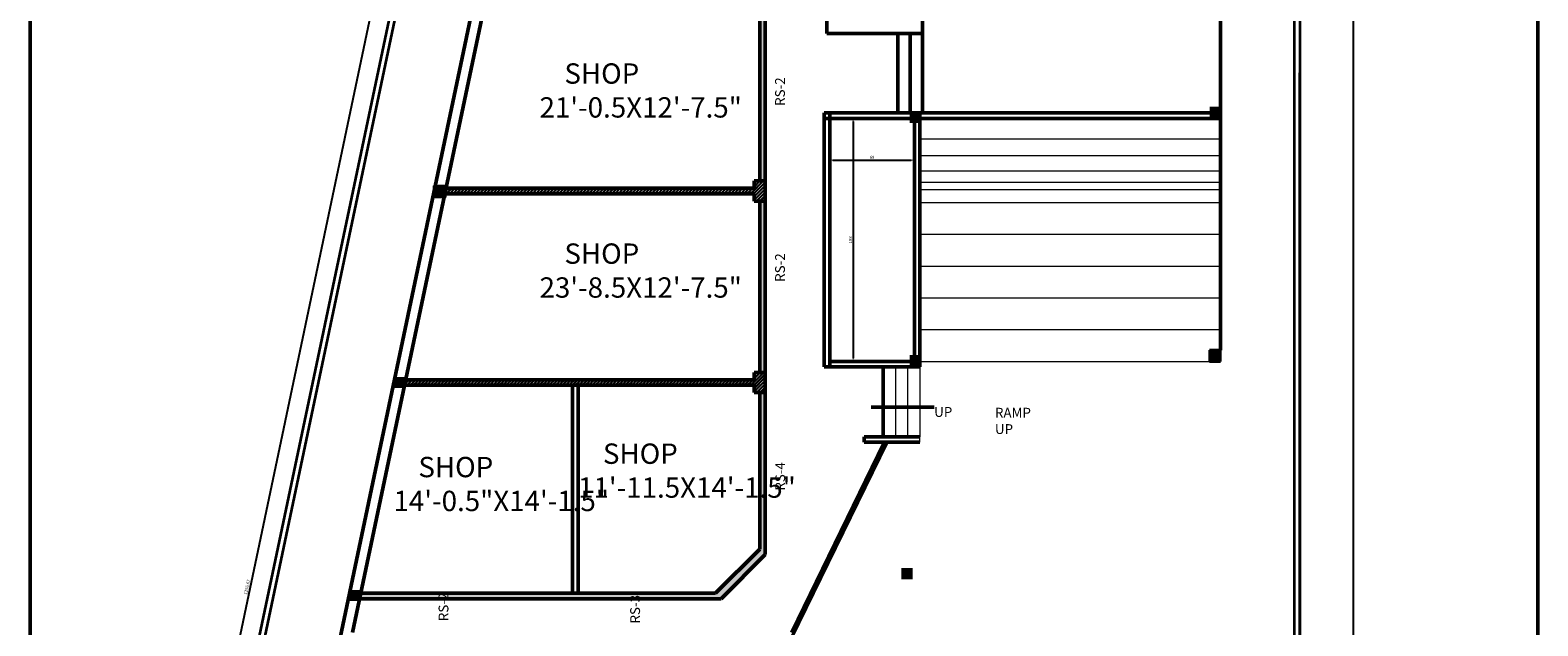
# Model space of a CAD drawing. Units: millimetres. Extents: x 2134 to 3363, y 1052 to 3233.
# Tile 5 of 11: x 2134 to 3363, y 1782 to 2268. Entities that reach past the tile are written whole.
import ezdxf

# ---------------------------------------------------------------- set-up
doc = ezdxf.new("R2010")
doc.units = ezdxf.units.MM
for name, color, linetype, lineweight in [('A-ANNO-DIMS', 2, 'Continuous', 18), ('A-ANNO-TEXT', 7, 'Continuous', 18), ('A-ANNO-TTLB', 7, 'Continuous', 50), ('A-AREA-IDEN', 3, 'Continuous', 18), ('A-COLS', 1, 'Continuous', 35), ('A-FLOR-STRS', 3, 'Continuous', 18), ('A-WALL', 7, 'Continuous', 50), ('A-WALL-PATT', 8, 'Continuous', 13), ('C-PROP', 6, 'Continuous', 35)]:
    doc.layers.add(name, color=color, linetype=linetype, lineweight=lineweight)
doc.styles.get("Standard").update_dxf_attribs({"font": 'arial.ttf'})
doc.styles.add('YQ_DIM', font='SUPEROS.SHX', dxfattribs={"width": 0.8, "bigfont": 'HZDX.SHX'})
doc.dimstyles.new('ISO-25', dxfattribs={"dimtxt": 2.5, "dimasz": 2.5, "dimexe": 1.25, "dimexo": 0.625, "dimtad": 1, "dimtxsty": 'Standard', "dimcen": 2.5, "dimadec": 0, "dimazin": 0, "dimtfac": 1, "dimtmove": 0, "dimatfit": 3, "dimfxl": 1, "dimarcsym": 0})

# ---------------------------------------------------------------- blocks, each defined once
blk = doc.blocks.new('*D8')
at = {"layer": 'A-ANNO-DIMS', "color": 0, "lineweight": -2, "transparency": 16777216}
for p, q in [((2442.4, 2425.8), (2184.5, 1201)), ((2457.7, 2425.1), (2441.7, 2428.5)), ((2198.8, 1195.4), (2182.8, 1198.8))]:
    blk.add_line(p, q, dxfattribs=at)
at = {"layer": 'A-ANNO-DIMS', "color": 0, "transparency": 16777216}
for points in [[(2442, 2425.9), (2442.8, 2425.7), (2442.9, 2428.3)], [(2184.1, 1201.1), (2185, 1200.9), (2184, 1198.5)]]:
    blk.add_solid(points, dxfattribs=at)
at = {"layer": 'Defpoints', "color": 0, "transparency": 16777216}
for p in [(2458.4, 2425), (2184, 1198.5), (2199.5, 1195.3)]:
    blk.add_point(p, dxfattribs=at)
at = {"layer": 'A-ANNO-DIMS', "color": 0, "transparency": 16777216, "insert": (2311.4, 1813.8), "char_height": 2.5, "attachment_point": 5, "rotation": 78.1108}
blk.add_mtext('1256,67', dxfattribs=at)
blk = doc.blocks.new('*D9')
at = {"layer": 'A-ANNO-DIMS', "color": 0, "lineweight": -2, "transparency": 16777216}
for p, q in [((3169.5, 3063.8), (3213.5, 3063.8)), ((3212.2, 3061.3), (3212.2, 1770.3)), ((3169.5, 1767.8), (3213.5, 1767.8))]:
    blk.add_line(p, q, dxfattribs=at)
at = {"layer": 'A-ANNO-DIMS', "color": 0, "transparency": 16777216}
for points in [[(3211.8, 3061.3), (3212.6, 3061.3), (3212.2, 3063.8)], [(3211.8, 1770.3), (3212.6, 1770.3), (3212.2, 1767.8)]]:
    blk.add_solid(points, dxfattribs=at)
at = {"layer": 'Defpoints', "color": 0, "transparency": 16777216}
for p in [(3168.8, 3063.8), (3168.8, 1767.8), (3212.2, 1767.8)]:
    blk.add_point(p, dxfattribs=at)
at = {"layer": 'A-ANNO-DIMS', "color": 0, "transparency": 16777216, "insert": (3210.3, 2415.8), "char_height": 2.5, "attachment_point": 5, "rotation": 90}
blk.add_mtext('1296', dxfattribs=at)
blk = doc.blocks.new('*D13')
at = {"layer": 'A-ANNO-DIMS', "color": 0, "lineweight": -2, "transparency": 16777216}
for p, q in [((2785.8, 2162.4), (2785.8, 2163)), ((2854.8, 2162.4), (2854.8, 2163)), ((2788.3, 2161.8), (2852.3, 2161.8))]:
    blk.add_line(p, q, dxfattribs=at)
at = {"layer": 'A-ANNO-DIMS', "color": 0, "transparency": 16777216}
for points in [[(2788.3, 2162.2), (2788.3, 2161.3), (2785.8, 2161.8)], [(2852.3, 2162.2), (2852.3, 2161.3), (2854.8, 2161.8)]]:
    blk.add_solid(points, dxfattribs=at)
at = {"layer": 'Defpoints', "color": 0, "transparency": 16777216}
for p in [(2785.8, 2161.8), (2854.8, 2161.8), (2854.8, 2161.8)]:
    blk.add_point(p, dxfattribs=at)
at = {"layer": 'A-ANNO-DIMS', "color": 0, "transparency": 16777216, "insert": (2820.3, 2163.7), "char_height": 2.5, "attachment_point": 5}
blk.add_mtext('69', dxfattribs=at)
blk = doc.blocks.new('*D14')
at = {"layer": 'A-ANNO-DIMS', "color": 0, "lineweight": -2, "transparency": 16777216}
for p, q in [((2804.4, 2195.8), (2806.2, 2195.8)), ((2804.9, 2193.3), (2804.9, 2000.3)), ((2809.9, 1997.8), (2803.7, 1997.8))]:
    blk.add_line(p, q, dxfattribs=at)
at = {"layer": 'A-ANNO-DIMS', "color": 0, "transparency": 16777216}
for points in [[(2804.5, 2193.3), (2805.3, 2193.3), (2804.9, 2195.8)], [(2804.5, 2000.3), (2805.3, 2000.3), (2804.9, 1997.8)]]:
    blk.add_solid(points, dxfattribs=at)
at = {"layer": 'Defpoints', "color": 0, "transparency": 16777216}
for p in [(2803.8, 2195.8), (2804.9, 1997.8), (2810.6, 1997.8)]:
    blk.add_point(p, dxfattribs=at)
at = {"layer": 'A-ANNO-DIMS', "color": 0, "transparency": 16777216, "insert": (2803, 2096.8), "char_height": 2.5, "attachment_point": 5, "rotation": 90}
blk.add_mtext('198', dxfattribs=at)
blk = doc.blocks.new('*D6')
at = {"layer": 'A-ANNO-DIMS', "color": 0, "lineweight": -2, "transparency": 16777216}
blk.add_arc((2458.4, 2425), 20.3, 94.064, 251.0467, dxfattribs=at)
at = {"layer": 'A-ANNO-DIMS', "color": 0, "transparency": 16777216}
for points in [[(2456.9, 2445.7), (2456.9, 2444.8), (2459.4, 2445.3)], [(2451.9, 2406.2), (2451.7, 2405.4), (2454.2, 2405.2)]]:
    blk.add_solid(points, dxfattribs=at)
at = {"layer": 'Defpoints', "color": 0, "transparency": 16777216}
for p in [(2491.8, 3063.8), (2441.9, 2436.9), (2458.4, 2425), (2458.4, 2425), (2197.1, 1183.9)]:
    blk.add_point(p, dxfattribs=at)
at = {"layer": 'A-ANNO-DIMS', "color": 0, "transparency": 16777216, "insert": (2436.4, 2427.9), "char_height": 2.5, "attachment_point": 5, "rotation": 82.5554}
blk.add_mtext('171°', dxfattribs=at)

msp = doc.modelspace()

# ---------------------------------------------------------------- hatches: boundary and pattern name
at = {"layer": 'A-COLS'}
h = msp.add_hatch(color=256, dxfattribs=at)
h.dxf.hatch_style = 1
h.paths.add_polyline_path([(2859.858, 2200.875), (2850.858, 2200.875), (2850.858, 2191.875), (2859.858, 2191.875)])
h = msp.add_hatch(color=256, dxfattribs=at)
h.dxf.hatch_style = 1
h.paths.add_polyline_path([(3104.339, 2205.375), (3095.339, 2205.375), (3095.339, 2196.375), (3104.339, 2196.375)])
h = msp.add_hatch(color=256, dxfattribs=at)
h.dxf.hatch_style = 1
h.paths.add_polyline_path([(2472.483, 2140.686), (2464.415, 2140.686), (2463.483, 2136.26), (2463.483, 2131.686), (2471.635, 2131.686), (2472.483, 2135.714)])
h = msp.add_hatch(color=256, dxfattribs=at)
h.dxf.hatch_style = 1
h.paths.add_polyline_path([(2859.858, 2002.875), (2850.858, 2002.875), (2850.858, 1993.875), (2859.858, 1993.875)])
h = msp.add_hatch(color=256, dxfattribs=at)
h.dxf.hatch_style = 1
h.paths.add_polyline_path([(3104.339, 2006.774), (3095.339, 2006.774), (3095.339, 1997.774), (3104.339, 1997.774)])
h = msp.add_hatch(color=256, dxfattribs=at)
h.dxf.hatch_style = 1
h.paths.add_polyline_path([(2440.045, 1985.133), (2431.045, 1985.133), (2431.045, 1976.133), (2440.045, 1976.133)])
h = msp.add_hatch(color=256, dxfattribs=at)
h.dxf.hatch_style = 1
h.paths.add_polyline_path([(2853.256, 1829.254), (2844.256, 1829.254), (2844.256, 1820.254), (2853.256, 1820.254)])
h = msp.add_hatch(color=256, dxfattribs=at)
h.dxf.hatch_style = 1
h.paths.add_polyline_path([(2403.25, 1811.556), (2394.25, 1811.556), (2394.25, 1802.556), (2403.25, 1802.556)])
at = {"layer": 'A-WALL-PATT'}
h = msp.add_hatch(color=256, dxfattribs=at)
h.dxf.hatch_style = 1
h.paths.add_polyline_path([(2733.282, 2279.774), (2728.782, 2279.774), (2728.782, 2144.774), (2733.282, 2144.774)])
h.paths.add_polyline_path([(2733.282, 2435.778), (2728.782, 2435.778), (2728.782, 2296.274), (2733.282, 2296.274)])
h.paths.add_polyline_path([(2733.282, 2128.274), (2728.782, 2128.274), (2728.782, 1988.794), (2733.282, 1988.794)])
h.paths.add_polyline_path([(2733.282, 1972.299), (2728.782, 1972.299), (2728.782, 1844.774), (2692.782, 1808.774), (2403.682, 1808.774), (2402.735, 1804.274), (2697.282, 1804.274), (2733.282, 1840.274)])
h.paths.add_polyline_path([(2733.282, 2591.847), (2728.782, 2591.847), (2728.782, 2452.274), (2733.282, 2452.276)])
h.paths.add_polyline_path([(2733.282, 2747.554), (2728.782, 2747.554), (2728.782, 2608.342), (2733.282, 2608.342)])
h.paths.add_polyline_path([(2733.282, 2843.718), (2728.782, 2843.718), (2728.782, 2764.049), (2733.282, 2764.049)])
h.paths.add_polyline_path([(2733.282, 3012.274), (2728.782, 3012.274), (2728.782, 2860.213), (2733.282, 2860.213)])
h = msp.add_hatch(dxfattribs=at)
h.set_pattern_fill('ANSI32', color=256, scale=0.2)
h.set_pattern_definition([(45, (2052.4981, 1503.6934), (-1.3470384, 1.3470384), []), (45, (2053.3961, 1503.6934), (-1.3470384, 1.3470384), [])])
h.paths.add_polyline_path([(2733.282, 2144.774), (2728.782, 2144.774), (2728.782, 2144.769), (2724.282, 2144.769), (2724.282, 2138.774), (2473.126, 2138.774), (2472.179, 2134.274), (2724.282, 2134.274), (2724.282, 2128.274), (2728.782, 2128.274), (2733.282, 2128.274)])
h.paths.add_polyline_path([(2733.282, 2608.342), (2724.282, 2608.342), (2724.282, 2602.274), (2541.252, 2602.274), (2541.016, 2597.774), (2724.282, 2597.774), (2724.282, 2591.847), (2733.282, 2591.847)])
h.paths.add_polyline_path([(2733.282, 2452.274), (2728.782, 2452.274), (2724.282, 2452.274), (2724.282, 2446.274), (2533.076, 2446.274), (2532.851, 2441.988), (2724.282, 2441.783), (2724.282, 2435.778), (2728.782, 2435.778), (2733.282, 2435.778)])
h.paths.add_polyline_path([(2733.282, 1988.794), (2724.282, 1988.794), (2724.282, 1982.774), (2440.298, 1982.774), (2439.351, 1978.274), (2724.282, 1978.274), (2724.282, 1972.299), (2733.282, 1972.299)])
h.paths.add_polyline_path([(2733.282, 2296.269), (2722.735, 2296.269), (2722.735, 2290.274), (2505.008, 2290.274), (2504.061, 2285.774), (2722.735, 2285.774), (2722.735, 2279.774), (2728.782, 2279.774), (2733.282, 2279.774)])

# ---------------------------------------------------------------- linework, layer by layer
at = {"layer": 'A-ANNO-TTLB', "ltscale": 0.5}
msp.add_lwpolyline([(2134.34, 3233.23), (3362.77, 3233.23), (3362.77, 1152.237), (2134.34, 1152.237)], close=True, dxfattribs=at)
at = {"layer": 'A-COLS'}
for p, q in [((3104.339, 2006.774), (3095.339, 2006.774)), ((3095.339, 2006.774), (3095.339, 1997.774)), ((3104.339, 1997.774), (3104.339, 2006.774)), ((3095.339, 1997.774), (3104.339, 1997.774))]:
    msp.add_line(p, q, dxfattribs=at)
msp.add_lwpolyline([(2463.483, 2140.686), (2472.483, 2140.686), (2472.483, 2131.686), (2463.483, 2131.686)], close=True, dxfattribs=at)
at = {"layer": 'A-FLOR-STRS'}
for p, q in [((2859.282, 2178.988), (3104.339, 2178.988)), ((2859.282, 2165.478), (3104.339, 2165.478)), ((2859.282, 2153.101), (3104.339, 2153.101)), ((2859.282, 2143.743), (3104.339, 2143.743)), ((3104.339, 2137.474), (2859.282, 2137.474)), ((2859.282, 2127.213), (3104.339, 2127.213)), ((2859.282, 2101.325), (3104.339, 2101.325)), ((2859.282, 2075.437), (3104.339, 2075.437)), ((2859.282, 2049.549), (3104.339, 2049.549)), ((2859.282, 2023.661), (3104.339, 2023.661)), ((2839.282, 1993.274), (2839.282, 1936.274)), ((2849.282, 1993.274), (2849.282, 1936.274)), ((2859.282, 1997.774), (3104.339, 1997.774)), ((2859.282, 1993.274), (2859.282, 1936.274)), ((2859.282, 1931.774), (2859.282, 1936.274))]:
    msp.add_line(p, q, dxfattribs=at)
at = {"layer": 'A-WALL'}
for p, q in [((2733.282, 3012.274), (2733.282, 1840.274)), ((3104.339, 3021.274), (3104.339, 2017.274)), ((3104.339, 3021.274), (3104.339, 2006.774)), ((2783.402, 2659.962), (2783.402, 2264.962)), ((2861.402, 2659.962), (2861.402, 2264.962)), ((2386.865, 1772.344), (2522.51, 2416.625)), ((2396.963, 1776.846), (2531.497, 2416.154)), ((2728.782, 2279.774), (2728.782, 2144.769)), ((2783.402, 2264.962), (2861.402, 2264.962)), ((2841.402, 2264.962), (2841.402, 2200.274)), ((2851.402, 2200.274), (2851.402, 2264.962)), ((2861.402, 2264.962), (2861.402, 2200.274)), ((2781.282, 2200.274), (3104.339, 2200.274)), ((2781.282, 2200.274), (2781.282, 1993.274)), ((2781.282, 2200.274), (2781.282, 2195.774)), ((2785.782, 2200.274), (2785.782, 1993.274)), ((2854.782, 2200.274), (2854.782, 1993.274)), ((2859.282, 2200.274), (2859.282, 1993.274)), ((2781.282, 2195.774), (3104.339, 2195.774)), ((2473.209, 2138.774), (2724.282, 2138.774)), ((2724.282, 2138.769), (2724.282, 2144.769)), ((2724.282, 2144.769), (2728.782, 2144.769)), ((2728.782, 2144.774), (2733.282, 2144.774)), ((3104.339, 2143.743), (3104.339, 2137.474)), ((2472.262, 2134.274), (2724.282, 2134.274)), ((2724.282, 2128.274), (2724.282, 2134.278)), ((2728.782, 2128.274), (2724.282, 2128.274)), ((2728.782, 2128.274), (2728.782, 1988.794)), ((2728.782, 2128.274), (2733.282, 2128.274)), ((2785.782, 1993.274), (2781.282, 1993.274)), ((2785.782, 1997.774), (2859.282, 1997.774)), ((2785.782, 1993.274), (2859.282, 1993.274)), ((2829.282, 1993.274), (2829.282, 1936.274)), ((2439.418, 1978.274), (2724.282, 1978.274)), ((2440.365, 1982.774), (2724.282, 1982.774)), ((2576.282, 1978.274), (2576.282, 1808.774)), ((2580.782, 1978.274), (2580.782, 1808.774)), ((2724.282, 1982.774), (2724.282, 1988.794)), ((2724.282, 1988.794), (2733.282, 1988.794)), ((2724.282, 1972.299), (2724.282, 1978.304)), ((2733.282, 1972.299), (2724.282, 1972.299)), ((2728.782, 1972.299), (2728.782, 1844.774)), ((2870.901, 1960.541), (2819.462, 1960.541)), ((2754.719, 1776.895), (2830.205, 1931.774)), ((2754.719, 1772.395), (2832.735, 1931.774)), ((2859.282, 1936.274), (2813.822, 1936.274)), ((2813.822, 1936.274), (2813.822, 1931.774)), ((2813.822, 1931.774), (2859.282, 1931.774)), ((2692.782, 1808.774), (2728.782, 1844.774)), ((2697.282, 1804.274), (2733.282, 1840.274)), ((2403.682, 1808.774), (2692.782, 1808.774)), ((2402.735, 1804.274), (2697.282, 1804.274))]:
    msp.add_line(p, q, dxfattribs=at)
at = {"layer": 'C-PROP'}
for p, q in [((3164.339, 3059.32), (3164.339, 1770.366)), ((3168.839, 3063.82), (3168.839, 1767.82)), ((2197.066, 1183.92), (2458.361, 2425.007)), ((2203.596, 1193.093), (2462.764, 2424.08)), ((3168.839, 1767.82), (3168.839, 2232.82))]:
    msp.add_line(p, q, dxfattribs=at)

# ---------------------------------------------------------------- texts
at = {"layer": 'A-ANNO-TEXT', "char_height": 8, "attachment_point": 1, "rotation": 90, "style": 'YQ_DIM'}
for s, insert in [('{\\fSwis721 BlkCn BT|b0|i0|c0|p34;RS-2}', (2741.318, 2205.935)), ('{\\fSwis721 BlkCn BT|b0|i0|c0|p34;RS-2}', (2741.318, 2062.545)), ('{\\fSwis721 BlkCn BT|b0|i0|c0|p34;RS-4}', (2741.445, 1892.345)), ('{\\fSwis721 BlkCn BT|b0|i0|c0|p34;RS-2}', (2467.134, 1786.016)), ('{\\fSwis721 BlkCn BT|b0|i0|c0|p34;RS-3}', (2623.242, 1784.103))]:
    msp.add_mtext_dynamic_manual_height_columns(s, width=14.9584, gutter_width=12.5, heights=[0], dxfattribs=dict(at, insert=insert))
at = {"layer": 'A-ANNO-TEXT', "char_height": 8, "attachment_point": 1, "style": 'YQ_DIM'}
for s, width, insert in [('{\\fSitka Banner Semibold|b1|i0|c0|p2;UP}', 3.68944, (2870.901, 1960.541)), ('{\\fSTZhongsong|b1|i0|c0|p2;RAMP UP}', 45.72976, (2920.422, 1959.911))]:
    msp.add_mtext_dynamic_manual_height_columns(s, width=width, gutter_width=12.5, heights=[0], dxfattribs=dict(at, insert=insert))
at = {"layer": 'A-AREA-IDEN', "char_height": 16.56819, "attachment_point": 1, "style": 'YQ_DIM'}
for s, insert in [('{\\f@SimSun|b1|i0|c0|p2; \\f@Arial Unicode MS|b1|i0|c0|p34;   SHOP\\P21\'-0.5X12\'-7.5\\f@SimSun|b1|i0|c0|p2;"}', (2549.381, 2240.611)), ('{\\f@SimSun|b1|i0|c0|p2; \\f@Arial Unicode MS|b1|i0|c0|p34;   SHOP\\P23\'-8.5X12\'-7.5\\f@SimSun|b1|i0|c0|p2;"}', (2549.381, 2093.844)), ('{\\f@SimSun|b1|i0|c0|p2; \\f@Arial Unicode MS|b1|i0|c0|p34;   SHOP\\P11\'-11.5X14\'-1.5\\f@SimSun|b1|i0|c0|p2;"}', (2580.782, 1930.818)), ('{\\f@SimSun|b1|i0|c0|p2; \\f@Arial Unicode MS|b1|i0|c0|p34;   SHOP\\P14\'-0.5"X14\'-1.5\\f@SimSun|b1|i0|c0|p2;"}', (2430.407, 1919.904))]:
    msp.add_mtext_dynamic_manual_height_columns(s, width=128.94034, gutter_width=26.518, heights=[0], dxfattribs=dict(at, insert=insert))

# ---------------------------------------------------------------- dimensions: what is measured, and where the dimension line sits
at = {"layer": 'A-ANNO-DIMS'}
dim = msp.add_angular_dim_2l(base=(2441.938, 2436.923), line1=((2197.066, 1183.92), (2458.361, 2425.007)), line2=((2458.361, 2425.007), (2491.839, 3063.82)), dimstyle='ISO-25', override={"dimclrd": 0, "dimclre": 0, "dimclrt": 0}, dxfattribs=at)
dim.commit()
dim.dimension.update_dxf_attribs({"geometry": '*D6', "text_midpoint": (2436.377, 2427.88)})
for base, p1, p2, picture, middle in [((3212.229, 1767.82), (3168.839, 3063.82), (3168.839, 1767.82), '*D9', (3210.327, 2415.82)), ((2804.93, 1997.774), (2803.804, 2195.774), (2810.559, 1997.774), '*D14', (2803.028, 2096.774))]:
    dim = msp.add_linear_dim(base=base, p1=p1, p2=p2, angle=90, dimstyle='ISO-25', override={"dimclrd": 0, "dimclre": 0, "dimclrt": 0}, dxfattribs=at)
    dim.commit()
    dim.dimension.update_dxf_attribs({"geometry": picture, "text_midpoint": middle})
dim = msp.add_aligned_dim(p1=(2458.361, 2425.007), p2=(2199.46, 1195.291), distance=-15.77, dimstyle='ISO-25', override={"dimclrd": 0, "dimclre": 0, "dimclrt": 0}, dxfattribs=at)
dim.commit()
dim.dimension.update_dxf_attribs({"geometry": '*D8', "text_midpoint": (2311.397, 1813.836)})
dim = msp.add_linear_dim(base=(2854.782, 2161.757), p1=(2785.782, 2161.757), p2=(2854.782, 2161.757), dimstyle='ISO-25', override={"dimclrd": 0, "dimclre": 0, "dimclrt": 0}, dxfattribs=at)
dim.commit()
dim.dimension.update_dxf_attribs({"geometry": '*D13', "text_midpoint": (2820.282, 2163.658)})

doc.saveas('drawing.dxf')
